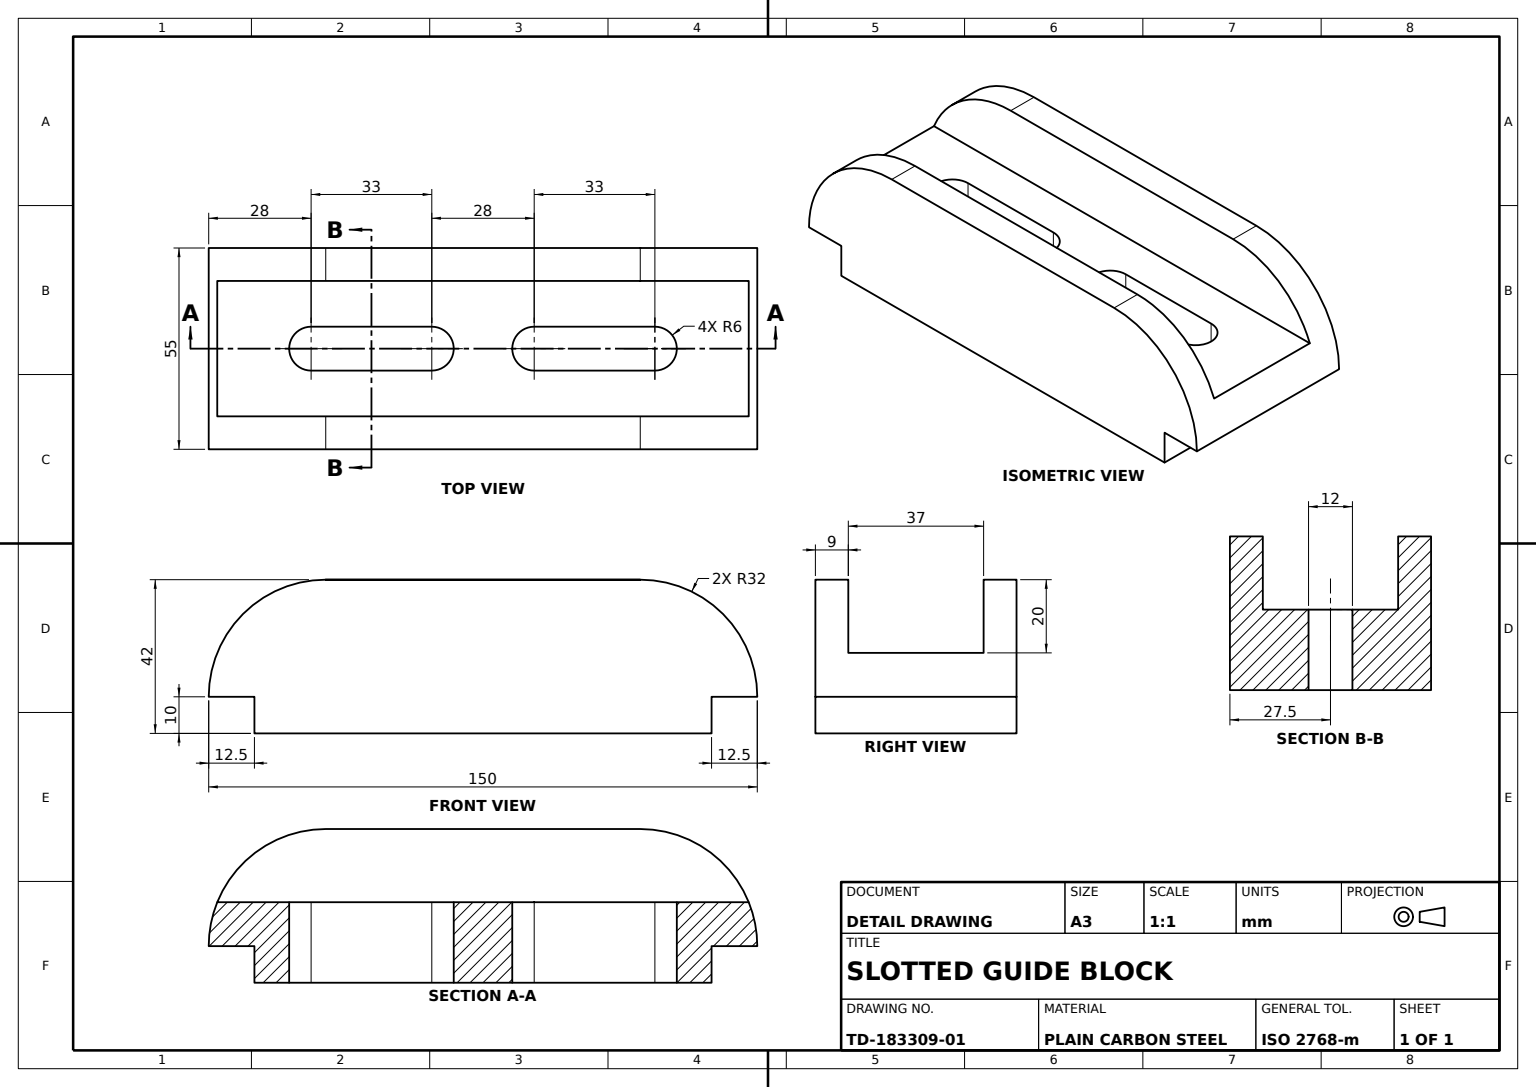
SolidWorks part; units mm, degrees
material "Plain Carbon Steel"
ref_plane "Front Plane" through (0, 0, 0) normal (0, 0, 1) x (1, 0, 0)
ref_plane "Top Plane" through (0, 0, 0) normal (0, 1, 0) x (1, 0, 0)
ref_plane "Right Plane" through (0, 0, 0) normal (1, 0, 0) x (0, 0, -1)
sketch "Block Profile Sketch" plane through (0, 0, 0) normal (0, 0, 1) x (1, 0, 0)
  line L0 (0, 0) -> (62.5, 0)
  line L1 (62.5, 0) -> (62.5, 10)
  line L3 (62.5, 10) -> (75, 10)
  line L5 (0, 42) -> (-43, 42)
  line L7 (0, 0) -> (-62.5, 0)
  line L8 (-62.5, 0) -> (-62.5, 10)
  line L9 (-62.5, 10) -> (-75, 10)
  line L10 (0, 42) -> (43, 42)
  arc A0 (-43, 42) -> (-75, 10) centre (-43, 10) ccw
  arc A1 (75, 10) -> (43, 42) centre (43, 10) ccw
  dimension "D9" = 43
  dimension "D2" = 32
  dimension "D5" = 32
  dimension "D1" = 42
  dimension "D3" = 32
  dimension "D4" = 62.5
  dimension "D6" = 32
  dimension "D7" = 62.5
  dimension "D8" = 42
  dimension "D10" = 43
extrude "Slide Block Body" add sketch "Block Profile Sketch" along normal mid plane 55
sketch "Centre Channel Sketch" plane through (0, 42, 0) normal (0, 1, 0) x (1, 0, 0)
  line L1 (0, 18.5) -> (92.6234, 18.5)
  line L2 (92.6234, 18.5) -> (92.6234, -18.5)
  line L3 (92.6234, -18.5) -> (-101.9901, -18.5)
  line L4 (-101.9901, -18.5) -> (-101.9901, 18.5)
  line L5 (-101.9901, 18.5) -> (0, 18.5)
  dimension "D1" = 194.6135
  dimension "D2" = 37
  dimension "D3" = 101.9901
  dimension "D4" = 18.5
  dimension "D5" = 18.5
extrude "Centre Channel 37 Wide" cut sketch "Centre Channel Sketch" against normal blind 20
sketch "Twin Slots Sketch" plane through (0, 22, 0) normal (0, 1, 0) x (1, 0, 0)
  line L0 (-72.6648, -18.5) -> (72.6648, -18.5) construction
  line L1 (-14, -6) -> (-47, -6)
  line L2 (14, 6) -> (47, 6)
  line L3 (14, -6) -> (47, -6)
  line L4 (-14, 6) -> (-47, 6)
  line L5 (43, 18.5) -> (-43, 18.5) construction
  arc A0 (14, 6) -> (14, -6) centre (14, 0) ccw
  arc A1 (47, -6) -> (47, 6) centre (47, 0) ccw
  arc A2 (-47, -6) -> (-47, 6) centre (-47, 0) cw
  arc A3 (-14, 6) -> (-14, -6) centre (-14, 0) cw
  dimension "D1" = 6
  dimension "D4" = 6
  dimension "D10" = 6
  dimension "D2" = 47
  dimension "D3" = 14
  dimension "D5" = 14
  dimension "D6" = 12.5
  dimension "D7" = 33
  dimension "D8" = 33
  dimension "D9" = 12.5
extrude "Twin Slots 2xR6" cut sketch "Twin Slots Sketch" against normal blind 38
